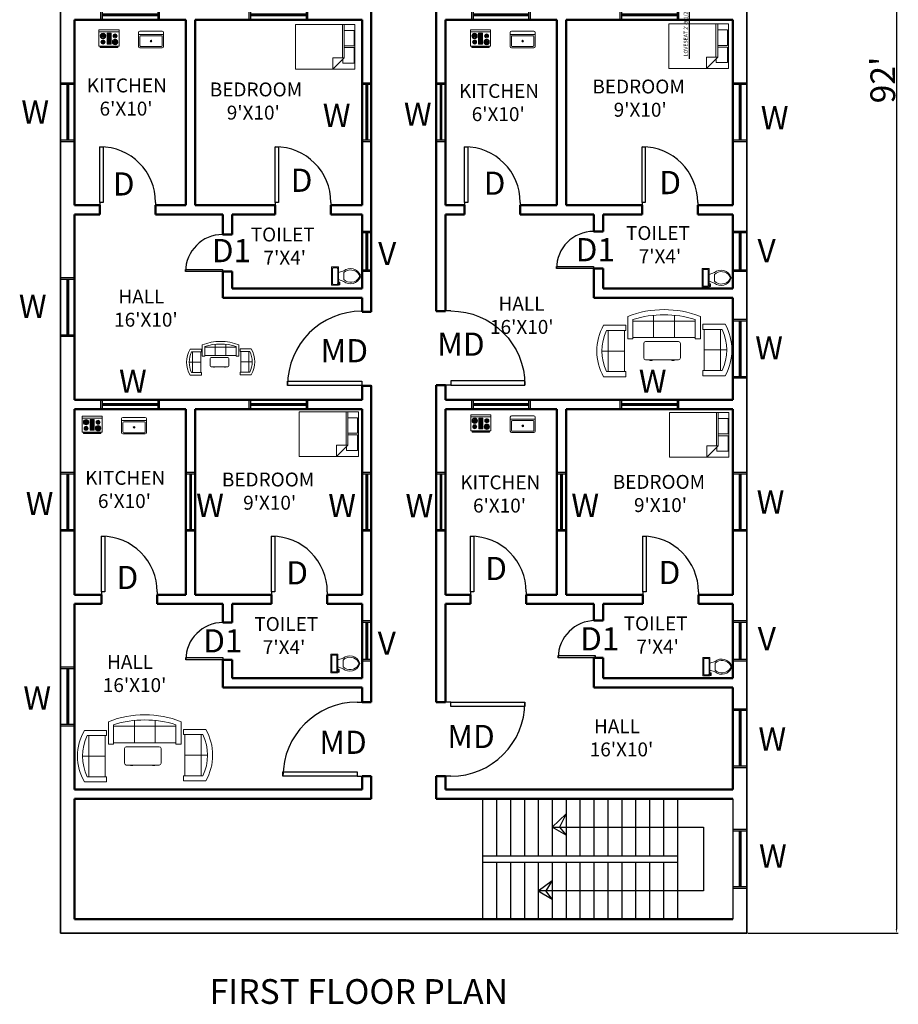
# Model space of a CAD drawing. Units: inches. Extents: x -25308 to -23933, y 10755 to 11996.
# Tile 1 of 6: x -25308 to -24739, y 10765 to 11402. Entities that reach past the tile are written whole.
import ezdxf

# ---------------------------------------------------------------- set-up
doc = ezdxf.new("R2010")
doc.units = ezdxf.units.IN
for name, color, linetype, lineweight in [('A-ANNO-DIMS', 2, 'Continuous', 18), ('A-ANNO-SYMB', 3, 'Continuous', 18), ('A-ANNO-TEXT', 7, 'Continuous', 25), ('A-AREA-IDEN', 7, 'Continuous', 18), ('A-DOOR', 3, 'Continuous', 25), ('A-FLOR-FIXT', 8, 'Continuous', 18), ('A-FLOR-STRS', 2, 'Continuous', 25), ('A-FURN', 8, 'Continuous', 18), ('A-GLAZ', 4, 'Continuous', 25), ('A-WALL', 7, 'Continuous', 50), ('C-PROP', 30, 'Continuous', 35)]:
    doc.layers.add(name, color=color, linetype=linetype, lineweight=lineweight)
doc.styles.get("Standard").update_dxf_attribs({"font": 'arial.ttf'})
doc.dimstyles.new('ISO-25', dxfattribs={"dimtxt": 2.5, "dimasz": 2.5, "dimexe": 1.25, "dimexo": 0.625, "dimtad": 1, "dimdec": 0, "dimlunit": 3, "dimtxsty": 'Standard', "dimcen": 2.5, "dimadec": 0, "dimazin": 0, "dimtfac": 1, "dimtdec": 0, "dimtmove": 0, "dimatfit": 3, "dimfxl": 1, "dimarcsym": 0})

# ---------------------------------------------------------------- blocks, each defined once
blk = doc.blocks.new('*U8')
for p, q in [((0, 0), (0, -100)), ((750, 0), (750, -100))]:
    blk.add_line(p, q)
blk.add_lwpolyline([(0, 0), (0, 750), (43.75, 750), (43.75, 0)], close=True)
blk.add_arc((0, 0), 750, 0, 90)
blk = doc.blocks.new('Desk - 30 x 60 in.')
for p, q in [((-26.999995, 0), (26.999995, 0)), ((-29.999995, -27), (-29.999995, -3)), ((29.999995, -3), (29.999995, -27)), ((26.999995, -30), (-26.999995, -30)), ((-20.000005, -30), (-20.000005, -31)), ((-20.000005, -31), (-16.000005, -31)), ((-16.000005, -31), (-16.000005, -30)), ((15.999995, -31), (15.999995, -30)), ((19.999995, -31), (15.999995, -31)), ((19.999995, -30), (19.999995, -31))]:
    blk.add_line(p, q)
for centre, start, end in [((-26.499995, -3.5), 98.1301, 171.8699), ((26.499995, -3.5), 8.130102, 81.8699), ((-26.499995, -26.5), 188.1301, 261.8699), ((26.499995, -26.5), 278.1301, 351.8699)]:
    blk.add_arc(centre, 3.535534, start, end)
blk = doc.blocks.new('Sofa - Roundback 7 ft.')
for p, q in [((-12.00002, -32.4421), (-12.00003, -6.5971)), ((11.99997, -32.4421), (11.99998, -6.5971)), ((-36.000027, -34), (-36.000027, -11.4696)), ((-35.999844, -13.3819), (35.9998, -13.3819)), ((35.99998, -34), (35.99998, -11.4696)), ((-36.000027, -32.4421), (35.99998, -32.4421))]:
    blk.add_line(p, q)
for points in [[(-36.000027, -34), (-42.000027, -34), (-42.000027, -8)], [(41.99998, -8), (41.99998, -34), (35.99998, -34)]]:
    blk.add_lwpolyline(points)
for centre, radius, start, end in [((0, -114.25), 114.25, 68.43141, 111.5686), ((-0.00001, -127.1968), 121.1968, 72.72033, 107.2797)]:
    blk.add_arc(centre, radius, start, end)
blk = doc.blocks.new('Sofa - Roundback Loveseat 5 ft.')
for p, q in [((-24, -33.99998), (-24, -11.46958)), ((0, -32.44198), (0, -5.99998)), ((24.00004, -33.99998), (24.00004, -11.46958)), ((-23.9998, -13.38178), (23.99986, -13.38178)), ((-24, -32.44198), (24.00004, -32.44198))]:
    blk.add_line(p, q)
for points in [[(-24, -33.99998), (-30, -33.99998), (-30, -7.99998)], [(30.00004, -7.99998), (30.00004, -33.99998), (24.00004, -33.99998)]]:
    blk.add_lwpolyline(points)
for centre, radius, start, end in [((0, -60.24998), 60.24998, 60.13715, 119.8628), ((0, -61.38438), 55.38444, 64.32083, 115.6792)]:
    blk.add_arc(centre, radius, start, end)
blk = doc.blocks.new('Bed - Queen')
for p, q in [((0, -80.00003), (0, 0)), ((0, 0), (59.99999, 0)), ((59.99999, 0), (59.99999, -80.00003)), ((7.99999, -1.2), (28.79998, -1.2)), ((7.99999, -14.4), (7.99999, -1.2)), ((28.79998, -1.2), (28.79998, -14.4)), ((31.19999, -1.2), (51.99999, -1.2)), ((31.19999, -14.4), (31.19999, -1.2)), ((51.99999, -1.2), (51.99999, -16.4)), ((0, -14.4), (44.8, -14.4)), ((44.8, -16.8), (0, -16.8)), ((59.99999, -29.6), (44.8, -14.4)), ((44.8, -14.4), (44.8, -29.6)), ((51.99999, -16.4), (46.79936, -16.4)), ((44.8, -29.6), (59.99999, -29.6)), ((59.99999, -80.00003), (0, -80.00003))]:
    blk.add_line(p, q)
blk = doc.blocks.new('Range-Oven - 30 in top')
for p, q in [((0, -3), (30, -3)), ((12, -6), (18, -6)), ((13, -20), (13, -6)), ((14, -6), (14, -20)), ((15, -20), (15, -6)), ((16, -6), (16, -20)), ((17, -20), (17, -6)), ((6, -24), (6, -25)), ((8, -25), (8, -24)), ((18, -20), (12, -20)), ((22, -25), (22, -24)), ((24, -24), (24, -25))]:
    blk.add_line(p, q)
for points in [[(0, -24), (0, 0), (30, 0), (30, -24)], [(12, -21), (12, -5), (18, -5), (18, -21)], [(2, -26), (2, -25), (28, -25), (28, -26)]]:
    blk.add_lwpolyline(points, close=True)
for centre, radius in [((6, -9), 4), ((6, -9), 3), ((6, -9), 2), ((6, -9), 1), ((24, -18), 4), ((24, -9), 3), ((24, -9), 2), ((24, -9), 1), ((6, -18), 3), ((6, -18), 2), ((6, -18), 1), ((24, -18), 3), ((24, -18), 2), ((24, -18), 1)]:
    blk.add_circle(centre, radius)
blk = doc.blocks.new('Sink-single - 30 in top')
blk.add_line((-15, -3.999996), (15, -3.999996))
for points in [[(-13.5, 0), (13.5, 0)], [(-15, -18.499996), (-15, -1.5)], [(-13.5, -17.499996), (-13.5, -6.499996)], [(-12.5, -5.499996), (12.5, -5.499996)], [(13.5, -6.499996), (13.5, -17.499996)], [(15, -1.5), (15, -18.499996)], [(13.5, -19.999996), (-13.5, -19.999996)], [(12.5, -18.499996), (-12.5, -18.499996)]]:
    blk.add_lwpolyline(points)
for radius in [1, 0.5]:
    blk.add_circle((0, -11.999996), radius)
for centre, radius, start, end in [((-13.5, -1.5), 1.5, 90, 180), ((-12.5, -6.499996), 1, 90, 180), ((12.5, -6.499996), 1, 0, 90), ((13.5, -1.5), 1.5, 0, 90), ((-13.5, -18.499996), 1.5, 180, 270), ((-12.5, -17.499996), 1, 180, 270), ((12.5, -17.499996), 1, 270, 0), ((13.5, -18.499996), 1.5, 270, 0)]:
    blk.add_arc(centre, radius, start, end)
blk = doc.blocks.new('Toilet - top')
for p, q in [((-10, -8.5), (-8, -8.5)), ((-10, -9.5), (-10, -8.5)), ((-7, -9.5), (-10, -9.5)), ((-8, -8.5), (-8, -8)), ((-7, -8), (-7, -9.5)), ((-4, -8), (-6, -14)), ((4, -8), (6, -14)), ((9.5, -6), (9.5, -2)), ((4, -14), (-4, -14))]:
    blk.add_line(p, q)
blk.add_lwpolyline([(10.5, -8), (10.5, 0), (-10.5, 0), (-10.5, -8)], close=True)
for points in [[(-9.5, -2), (-9.5, -6)], [(8.5, -1), (-8.5, -1)], [(-8.5, -7), (8.5, -7)]]:
    blk.add_lwpolyline(points)
for centre, radius, start, end in [((-8.6, -1.9), 0.884, 81.8699, 188.1301), ((-8.6, -6.1), 0.884, 171.8699, 278.1301), ((8.6, -1.9), 0.884, 351.8699, 98.1301), ((8.6, -6.1), 0.884, 261.8699, 8.1301), ((3.5, -21.6), 12.2, 141.4691, 247.9714), ((4.2, -21.8), 11.3, 136.3677, 238.9468), ((-3.5, -21.6), 12.2, 292.0284, 38.5307), ((-4.2, -21.8), 11.3, 301.053, 43.6321), ((0, -27.9), 4, 245.7318, 294.2682), ((0, -29), 4, 254.8605, 285.1395)]:
    blk.add_arc(centre, radius, start, end)
blk = doc.blocks.new('*D161')
at = {"layer": 'A-ANNO-DIMS', "color": 0, "lineweight": -2, "transparency": 16777216}
for p, q in [((-24836.82, 11915.12), (-24739.49, 11915.12)), ((-24740.74, 11912.62), (-24740.74, 10813.62)), ((-24836.82, 10811.12), (-24739.49, 10811.12))]:
    blk.add_line(p, q, dxfattribs=at)
at = {"layer": 'A-ANNO-DIMS', "color": 0, "transparency": 16777216}
for points in [[(-24741.15, 11912.62), (-24740.32, 11912.62), (-24740.74, 11915.12)], [(-24741.15, 10813.62), (-24740.32, 10813.62), (-24740.74, 10811.12)]]:
    blk.add_solid(points, dxfattribs=at)
at = {"layer": 'Defpoints', "color": 0, "transparency": 16777216}
for p in [(-24837.44, 11915.12), (-24837.44, 10811.12), (-24740.74, 10811.12)]:
    blk.add_point(p, dxfattribs=at)
at = {"layer": 'A-ANNO-DIMS', "color": 0, "transparency": 16777216, "insert": (-24749.53, 11363.12), "char_height": 2.5, "attachment_point": 5, "rotation": 90}
blk.add_mtext("{\\H6.4x;92'}", dxfattribs=at)
blk = doc.blocks.new('WIN-36-9IN')
for p, q in [((0, 9), (0, 0)), ((1, 9), (1, 0)), ((37, 9), (37, 0)), ((38, 9), (38, 0)), ((1, 5), (37, 5)), ((1, 4.5), (37, 4.5)), ((1, 4), (37, 4))]:
    blk.add_line(p, q)
blk = doc.blocks.new('VENT-24')
for p, q in [((0, 26), (9, 26)), ((0, 25), (9, 25)), ((4, 1), (4, 25)), ((4.5, 1), (4.5, 25)), ((5, 1), (5, 25)), ((0, 1), (9, 1)), ((0, 0), (9, 0))]:
    blk.add_line(p, q)
blk = doc.blocks.new('WIN-24-6IN')
for p, q in [((0, 26), (6, 26)), ((0, 25), (6, 25)), ((2.5, 1), (2.5, 25)), ((3, 1), (3, 25)), ((3.5, 1), (3.5, 25)), ((0, 1), (6, 1)), ((0, 0), (6, 0))]:
    blk.add_line(p, q)
blk = doc.blocks.new('WIN-36-6IN')
for p, q in [((0, 6), (0, 0)), ((1, 6), (1, 0)), ((1, 3.5), (37, 3.5)), ((1, 3), (37, 3)), ((1, 2.5), (37, 2.5)), ((37, 6), (37, 0)), ((38, 6), (38, 0))]:
    blk.add_line(p, q)
blk = doc.blocks.new('*D190')
at = {"layer": 'A-ANNO-DIMS', "color": 0, "lineweight": -2, "transparency": 16777216}
for p, q in [((-24870.41, 11454.17), (-24876.03, 11454.17)), ((-24874.78, 11451.67), (-24874.78, 11423.35)), ((-24870.41, 11420.85), (-24876.03, 11420.85)), ((-24874.78, 11420.85), (-24874.78, 11376.73))]:
    blk.add_line(p, q, dxfattribs=at)
at = {"layer": 'A-ANNO-DIMS', "color": 0, "transparency": 16777216}
for points in [[(-24875.2, 11451.67), (-24874.36, 11451.67), (-24874.78, 11454.17)], [(-24875.2, 11423.35), (-24874.36, 11423.35), (-24874.78, 11420.85)]]:
    blk.add_solid(points, dxfattribs=at)
at = {"layer": 'Defpoints', "color": 0, "transparency": 16777216}
for p in [(-24869.78, 11454.17), (-24874.78, 11420.85), (-24869.78, 11420.85)]:
    blk.add_point(p, dxfattribs=at)
at = {"layer": 'A-ANNO-DIMS', "color": 0, "transparency": 16777216, "insert": (-24876.7, 11397.54), "char_height": 2.5, "attachment_point": 5, "rotation": 90}
blk.add_mtext('LOVESEAT 2\'-9 1/2" TYP.', dxfattribs=at)

msp = doc.modelspace()

# ---------------------------------------------------------------- linework, layer by layer
at = {"layer": 'A-FLOR-STRS'}
for p, q in [((-25008.44, 10898.12), (-25008.44, 10820.12)), ((-24999.44, 10898.12), (-24999.44, 10861.12)), ((-24990.44, 10898.12), (-24990.44, 10861.12)), ((-24981.44, 10898.12), (-24981.44, 10861.12)), ((-24972.44, 10898.12), (-24972.44, 10861.12)), ((-24963.44, 10898.12), (-24963.44, 10861.12)), ((-24954.44, 10898.12), (-24954.44, 10861.12)), ((-24945.44, 10898.12), (-24945.44, 10861.12)), ((-24936.44, 10898.12), (-24936.44, 10861.12)), ((-24927.44, 10898.12), (-24927.44, 10861.12)), ((-24918.44, 10898.12), (-24918.44, 10861.12)), ((-24909.44, 10898.12), (-24909.44, 10861.12)), ((-24900.44, 10898.12), (-24900.44, 10861.12)), ((-24891.44, 10898.12), (-24891.44, 10861.12)), ((-24882.44, 10898.12), (-24882.44, 10820.12)), ((-24846.44, 10898.12), (-24846.44, 10820.12)), ((-24963.44, 10879.62), (-24954.44, 10888.37)), ((-24954.44, 10888.37), (-24958.64, 10879.62)), ((-24963.44, 10879.62), (-24865.43, 10879.62)), ((-24954.44, 10874.42), (-24963.44, 10879.62)), ((-24958.64, 10879.62), (-24954.44, 10874.42)), ((-24865.43, 10879.62), (-24865.43, 10838.62)), ((-25008.44, 10861.12), (-24882.44, 10861.12)), ((-25008.44, 10857.12), (-24882.44, 10857.12)), ((-24999.44, 10857.12), (-24999.44, 10820.12)), ((-24990.44, 10857.12), (-24990.44, 10820.12)), ((-24981.44, 10857.12), (-24981.44, 10820.12)), ((-24972.44, 10857.12), (-24972.44, 10820.12)), ((-24963.44, 10857.12), (-24963.44, 10820.12)), ((-24954.44, 10857.12), (-24954.44, 10820.12)), ((-24945.44, 10857.12), (-24945.44, 10820.12)), ((-24936.44, 10857.12), (-24936.44, 10820.12)), ((-24927.44, 10857.12), (-24927.44, 10820.12)), ((-24918.44, 10857.12), (-24918.44, 10820.12)), ((-24909.44, 10857.12), (-24909.44, 10820.12)), ((-24900.44, 10857.12), (-24900.44, 10820.12)), ((-24891.44, 10857.12), (-24891.44, 10820.12)), ((-24972.44, 10838.62), (-24963.44, 10845.13)), ((-24963.44, 10845.13), (-24967.58, 10838.62)), ((-24865.43, 10838.62), (-24972.44, 10838.62)), ((-24972.44, 10838.62), (-24963.44, 10833.02)), ((-24963.44, 10833.02), (-24967.58, 10838.62))]:
    msp.add_line(p, q, dxfattribs=at)
at = {"layer": 'A-WALL'}
for p, q in [((-25080.44, 11213.16), (-25080.44, 11416.06)), ((-25038.44, 11416.36), (-25038.44, 11213.64)), ((-25272.44, 11402.12), (-25200.44, 11402.12)), ((-25272.44, 11282.12), (-25272.44, 11402.12)), ((-25200.44, 11282.12), (-25200.44, 11402.12)), ((-25194.44, 11282.12), (-25194.44, 11402.12)), ((-25194.44, 11402.12), (-25086.44, 11402.12)), ((-25086.44, 11282.12), (-25086.44, 11402.12)), ((-25032.44, 11402.12), (-24960.44, 11402.12)), ((-25032.44, 11402.12), (-25032.44, 11282.12)), ((-24960.44, 11402.12), (-24960.44, 11282.12)), ((-24954.44, 11402.12), (-24954.44, 11282.12)), ((-24954.44, 11402.12), (-24846.44, 11402.12)), ((-24846.44, 11402.12), (-24846.44, 11282.12)), ((-25272.44, 11282.12), (-25256.02, 11282.12)), ((-25256.02, 11282.12), (-25256.02, 11276.12)), ((-25220.02, 11282.12), (-25220.02, 11276.12)), ((-25220.02, 11282.12), (-25200.44, 11282.12)), ((-25194.44, 11282.12), (-25142.59, 11282.12)), ((-25142.59, 11282.12), (-25142.59, 11276.12)), ((-25106.59, 11282.12), (-25106.59, 11276.12)), ((-25106.59, 11282.12), (-25086.44, 11282.12)), ((-25032.44, 11282.12), (-25020.09, 11282.12)), ((-25020.09, 11282.12), (-25020.09, 11276.12)), ((-24984.09, 11282.12), (-24984.09, 11276.12)), ((-24984.09, 11282.12), (-24960.44, 11282.12)), ((-24954.44, 11282.12), (-24905.28, 11282.12)), ((-24905.28, 11282.12), (-24905.28, 11276.12)), ((-24869.28, 11282.12), (-24869.28, 11276.12)), ((-24869.28, 11282.12), (-24846.44, 11282.12)), ((-25272.44, 11276.12), (-25256.02, 11276.12)), ((-25272.44, 11156.12), (-25272.44, 11276.12)), ((-25220.02, 11276.12), (-25176.44, 11276.12)), ((-25176.44, 11263.13), (-25176.44, 11276.12)), ((-25176.44, 11263.13), (-25176.44, 11276.12)), ((-25170.44, 11276.12), (-25142.59, 11276.12)), ((-25170.44, 11263.13), (-25170.44, 11276.12)), ((-25170.44, 11263.13), (-25170.44, 11276.12)), ((-25106.59, 11276.12), (-25086.44, 11276.12)), ((-25086.44, 11228.12), (-25086.44, 11276.12)), ((-25032.44, 11276.12), (-25020.09, 11276.12)), ((-25032.44, 11276.12), (-25032.44, 11213.64)), ((-24984.09, 11276.12), (-24936.44, 11276.12)), ((-24936.44, 11276.12), (-24936.44, 11265.12)), ((-24936.44, 11276.12), (-24936.44, 11265.12)), ((-24930.44, 11276.12), (-24930.44, 11265.12)), ((-24930.44, 11276.12), (-24930.44, 11265.12)), ((-24930.44, 11276.12), (-24905.28, 11276.12)), ((-24869.28, 11276.12), (-24846.44, 11276.12)), ((-24846.44, 11276.12), (-24846.44, 11228.12)), ((-25176.44, 11263.13), (-25170.44, 11263.13)), ((-24936.44, 11265.12), (-24930.44, 11265.12)), ((-25176.44, 11222.12), (-25176.44, 11239.13)), ((-25176.44, 11222.12), (-25176.44, 11239.13)), ((-25176.44, 11239.13), (-25170.44, 11239.13)), ((-25170.44, 11228.12), (-25170.44, 11239.13)), ((-25170.44, 11228.12), (-25170.44, 11239.13)), ((-24936.44, 11241.12), (-24930.44, 11241.12)), ((-24936.44, 11241.12), (-24936.44, 11222.12)), ((-24936.44, 11241.12), (-24936.44, 11222.12)), ((-24930.44, 11241.12), (-24930.44, 11228.12)), ((-24930.44, 11241.12), (-24930.44, 11228.12)), ((-25170.44, 11228.12), (-25086.44, 11228.12)), ((-24930.44, 11228.12), (-24846.44, 11228.12)), ((-25176.44, 11222.12), (-25086.44, 11222.12)), ((-25086.44, 11213.16), (-25086.44, 11222.12)), ((-24936.44, 11222.12), (-24846.44, 11222.12)), ((-24846.44, 11222.12), (-24846.44, 11156.12)), ((-25086.44, 11213.16), (-25080.44, 11213.16)), ((-25038.44, 11213.64), (-25032.44, 11213.64)), ((-25086.44, 11156.12), (-25086.44, 11165.16)), ((-25086.44, 11165.16), (-25080.44, 11165.16)), ((-25080.44, 10960.62), (-25080.44, 11165.16)), ((-25038.44, 11165.64), (-25032.44, 11165.64)), ((-25038.44, 11165.64), (-25038.44, 10960.62)), ((-25032.44, 11165.64), (-25032.44, 11156.12)), ((-25272.44, 11156.12), (-25176.44, 11156.12)), ((-25176.44, 11156.12), (-25086.44, 11156.12)), ((-25032.44, 11156.12), (-24846.44, 11156.12)), ((-25272.44, 11150.12), (-25200.44, 11150.12)), ((-25272.44, 11030.12), (-25272.44, 11150.12)), ((-25200.44, 11030.12), (-25200.44, 11150.12)), ((-25194.44, 11030.12), (-25194.44, 11150.12)), ((-25194.44, 11150.12), (-25086.44, 11150.12)), ((-25086.44, 11030.12), (-25086.44, 11150.12)), ((-25032.44, 11150.12), (-24960.44, 11150.12)), ((-25032.44, 11150.12), (-25032.44, 11030.12)), ((-24960.44, 11150.12), (-24960.44, 11030.12)), ((-24954.44, 11150.12), (-24954.44, 11030.12)), ((-24954.44, 11150.12), (-24846.44, 11150.12)), ((-24846.44, 11150.12), (-24846.44, 11030.12)), ((-25272.44, 11030.12), (-25254.98, 11030.12)), ((-25254.98, 11030.12), (-25254.98, 11024.12)), ((-25218.98, 11030.12), (-25218.98, 11024.12)), ((-25218.98, 11030.12), (-25200.44, 11030.12)), ((-25194.44, 11030.12), (-25144.93, 11030.12)), ((-25144.93, 11030.12), (-25144.93, 11024.12)), ((-25108.93, 11030.12), (-25108.93, 11024.12)), ((-25108.93, 11030.12), (-25086.44, 11030.12)), ((-25032.44, 11030.12), (-25016.19, 11030.12)), ((-25016.19, 11030.12), (-25016.19, 11024.12)), ((-24980.19, 11030.12), (-24980.19, 11024.12)), ((-24980.19, 11030.12), (-24960.44, 11030.12)), ((-24954.44, 11030.12), (-24904.78, 11030.12)), ((-24904.78, 11030.12), (-24904.78, 11024.12)), ((-24868.78, 11030.12), (-24868.78, 11024.12)), ((-24868.78, 11030.12), (-24846.44, 11030.12)), ((-25272.44, 11024.12), (-25254.98, 11024.12)), ((-25272.44, 10904.12), (-25272.44, 11024.12)), ((-25218.98, 11024.12), (-25176.44, 11024.12)), ((-25176.44, 11012.07), (-25176.44, 11024.12)), ((-25170.44, 11024.12), (-25144.93, 11024.12)), ((-25170.44, 11012.07), (-25170.44, 11024.12)), ((-25108.93, 11024.12), (-25086.44, 11024.12)), ((-25086.44, 10976.12), (-25086.44, 11024.12)), ((-25032.44, 11024.12), (-25016.19, 11024.12)), ((-25032.44, 11024.12), (-25032.44, 10960.62)), ((-24980.19, 11024.12), (-24936.44, 11024.12)), ((-24936.44, 11024.12), (-24936.44, 11013.36)), ((-24930.44, 11024.12), (-24930.44, 11013.36)), ((-24930.44, 11024.12), (-24904.78, 11024.12)), ((-24868.78, 11024.12), (-24846.44, 11024.12)), ((-24846.44, 11024.12), (-24846.44, 10976.12)), ((-25176.44, 11012.07), (-25170.44, 11012.07)), ((-24936.44, 11013.36), (-24930.44, 11013.36)), ((-24936.44, 10989.36), (-24930.44, 10989.36)), ((-24936.44, 10989.36), (-24936.44, 10970.12)), ((-24930.44, 10989.36), (-24930.44, 10976.12)), ((-25176.44, 10970.12), (-25176.44, 10988.07)), ((-25176.44, 10988.07), (-25170.44, 10988.07)), ((-25170.44, 10976.12), (-25170.44, 10988.07)), ((-25170.44, 10976.12), (-25086.44, 10976.12)), ((-24930.44, 10976.12), (-24846.44, 10976.12)), ((-25176.44, 10970.12), (-25086.44, 10970.12)), ((-25086.44, 10960.62), (-25086.44, 10970.12)), ((-24936.44, 10970.12), (-24846.44, 10970.12)), ((-24846.44, 10970.12), (-24846.44, 10904.12)), ((-25086.44, 10960.62), (-25080.44, 10960.62)), ((-25038.44, 10960.62), (-25032.44, 10960.62)), ((-25086.44, 10904.12), (-25086.44, 10912.62)), ((-25086.44, 10912.62), (-25080.44, 10912.62)), ((-25080.44, 10898.12), (-25080.44, 10912.62)), ((-25038.44, 10912.62), (-25032.44, 10912.62)), ((-25038.44, 10912.62), (-25038.44, 10898.12)), ((-25032.44, 10912.62), (-25032.44, 10904.12)), ((-25272.44, 10904.12), (-25086.44, 10904.12)), ((-25032.44, 10904.12), (-24846.44, 10904.12)), ((-25272.44, 10820.12), (-25272.44, 10898.12)), ((-25272.44, 10898.12), (-25080.44, 10898.12)), ((-25038.44, 10898.12), (-24846.44, 10898.12)), ((-24846.44, 10820.12), (-25272.44, 10820.12))]:
    msp.add_line(p, q, dxfattribs=at)
at = {"layer": 'C-PROP'}
for p, q in [((-25281.44, 10811.12), (-25281.44, 11915.12)), ((-24837.44, 11915.12), (-24837.44, 10811.12)), ((-24837.44, 10811.12), (-25281.44, 10811.12))]:
    msp.add_line(p, q, dxfattribs=at)

# ---------------------------------------------------------------- block references
at = {"layer": 'A-DOOR', "xscale": 0.0480000000000013, "yscale": 0.0480000000000013, "zscale": 0.0480000000000013}
for p in [(-25256.02, 11283.92), (-25142.59, 11283.92), (-25020.09, 11283.92), (-24905.28, 11283.92), (-25254.98, 11031.92), (-25144.93, 11031.92), (-25016.19, 11031.92), (-24904.78, 11031.92)]:
    msp.add_blockref('*U8', p, dxfattribs=at)
at = {"layer": 'A-DOOR'}
for p, xscale, yscale, zscale, rotation in [((-25176.62, 11239.14), 0.0320000000000009, 0.0320000000000009, 0.0320000000000009, 90), ((-24936.64, 11241.11), 0.0320000000000009, 0.0320000000000009, 0.0320000000000009, 90), ((-25086.6, 11165.52), 0.0640305237838995, 0.0640305237838995, 0.0640305237838995, 90), ((-25029.04, 11165.64), -0.0640305237838995, 0.0640305237838995, 0.0640305237838995, 270), ((-25176.44, 10988.07), 0.0320000000000009, 0.0320000000000009, 0.0320000000000009, 90), ((-24935.52, 10989.36), 0.0320000000000009, 0.0320000000000009, 0.0320000000000009, 90), ((-25089.54, 10912.6), 0.0640725944084254, 0.0640725944084254, 0.0640725944084254, 90), ((-25029.04, 10960.62), 0.0639999974380737, 0.0639999974380737, 0.0639999974380737, 270)]:
    msp.add_blockref('*U8', p, dxfattribs=dict(at, xscale=xscale, yscale=yscale, zscale=zscale, rotation=rotation))
at = {"layer": 'A-FLOR-FIXT'}
for name, p, xscale, yscale, zscale in [('Range-Oven - 30 in top', (-25256.64, 11395.48), 0.4338097128947254, 0.4338097128947254, 0.4338097128947254), ('Sink-single - 30 in top', (-25222.96, 11394.71), 0.5374838416175965, 0.5374838416175965, 0.5374838416175965), ('Range-Oven - 30 in top', (-25016.25, 11395.48), 0.4338097128947254, 0.4338097128947254, 0.4338097128947254), ('Sink-single - 30 in top', (-24982.57, 11394.71), 0.5374838416175965, 0.5374838416175965, 0.5374838416175965), ('Range-Oven - 30 in top', (-25267.61, 11145.62), 0.4338097128947254, 0.4338097128947254, 0.4338097128947254), ('Sink-single - 30 in top', (-25233.93, 11144.85), 0.5374838416175965, 0.5374838416175965, 0.5374838416175965), ('Range-Oven - 30 in top', (-25016.13, 11146.55), 0.4338097128947254, 0.4338097128947254, 0.4338097128947254), ('Sink-single - 30 in top', (-24982.45, 11145.78), 0.5374838416175965, 0.5374838416175965, 0.5374838416175965)]:
    msp.add_blockref(name, p, dxfattribs=dict(at, xscale=xscale, yscale=yscale, zscale=zscale))
at = {"layer": 'A-FLOR-FIXT', "xscale": 0.5659332238665749, "yscale": 0.5659332238665749, "zscale": 0.5659332238665749, "rotation": 90}
for p in [(-25106.15, 11236.21), (-24866.36, 11235.11), (-25106.64, 10985.6), (-24865.9, 10983.53)]:
    msp.add_blockref('Toilet - top', p, dxfattribs=at)
at = {"layer": 'A-FURN'}
for name, p, xscale, yscale, zscale, rotation in [('Bed - Queen', (-25091.03, 11399.04), 0.4812808282186369, 0.4812808282186369, 0.4812808282186369, 270), ('Bed - Queen', (-24849.37, 11399.35), 0.4812808282186369, 0.4812808282186369, 0.4812808282186369, 270), ('Sofa - Roundback Loveseat 5 ft.', (-24934.58, 11187.77), 0.5553292889469988, 0.5553292889469988, 0.5553292889469988, 89.99999999999999), ('Sofa - Roundback Loveseat 5 ft.', (-24847.12, 11188.42), 0.5553292889469988, 0.5553292889469988, 0.5553292889469988, 270), ('Sofa - Roundback Loveseat 5 ft.', (-25199.93, 11180.48), 0.2798473955820579, 0.2798473955820579, 0.2798473955820579, 89.99999999999999), ('Sofa - Roundback Loveseat 5 ft.', (-25155.86, 11180.81), 0.2798473955820579, 0.2798473955820579, 0.2798473955820579, 270), ('Bed - Queen', (-25088.71, 11148.46), 0.4812808282186369, 0.4812808282186369, 0.4812808282186369, 270), ('Bed - Queen', (-24849.08, 11147.95), 0.4812808282186369, 0.4812808282186369, 0.4812808282186369, 270), ('Sofa - Roundback Loveseat 5 ft.', (-25270.55, 10925.64), 0.5553292889469988, 0.5553292889469988, 0.5553292889469988, 89.99999999999999), ('Sofa - Roundback Loveseat 5 ft.', (-25183.09, 10926.28), 0.5553292889469988, 0.5553292889469988, 0.5553292889469988, 270)]:
    msp.add_blockref(name, p, dxfattribs=dict(at, xscale=xscale, yscale=yscale, zscale=zscale, rotation=rotation))
for name, p, xscale, yscale, zscale in [('Sofa - Roundback 7 ft.', (-24891.06, 11214.57), 0.559663641165008, 0.559663641165008, 0.559663641165008), ('Sofa - Roundback 7 ft.', (-25178, 11193.99), 0.2820316080914415, 0.2820316080914415, 0.2820316080914415), ('Desk - 30 x 60 in.', (-24892.36, 11193.91), 0.3949565101416468, 0.3949565101416468, 0.3949565101416468), ('Desk - 30 x 60 in.', (-25178.66, 11183.58), 0.1990306524997052, 0.1990306524997052, 0.1990306524997052), ('Sofa - Roundback 7 ft.', (-25227.03, 10952.43), 0.559663641165008, 0.559663641165008, 0.559663641165008), ('Desk - 30 x 60 in.', (-25228.33, 10931.77), 0.3949565101416468, 0.3949565101416468, 0.3949565101416468)]:
    msp.add_blockref(name, p, dxfattribs=dict(at, xscale=xscale, yscale=yscale, zscale=zscale))
at = {"layer": 'A-GLAZ'}
for name, p, rotation in [('WIN-36-6IN', (-25217.44, 11408.12), 180), ('WIN-36-6IN', (-25121.44, 11408.12), 180), ('WIN-36-6IN', (-24977.44, 11408.12), 180), ('WIN-36-6IN', (-24881.44, 11408.12), 180), ('WIN-36-9IN', (-25281.44, 11361.12), 270.0000000000339), ('WIN-36-6IN', (-25086.44, 11361.12), 270.0000000000161), ('WIN-36-6IN', (-25038.44, 11361.12), 270.0000000000268), ('WIN-36-9IN', (-24846.44, 11361.12), 270.0000000000198), ('WIN-24-6IN', (-25080.44, 11265.12), 180), ('VENT-24', (-24837.44, 11265.12), 180), ('VENT-24', (-24837.44, 11265.12), 180), ('WIN-36-9IN', (-25281.44, 11235.12), 270.0000000000315), ('WIN-36-9IN', (-24846.44, 11208.12), 270.0000000000173), ('WIN-36-6IN', (-25217.44, 11156.12), 180), ('WIN-36-6IN', (-25121.44, 11156.12), 180), ('WIN-36-6IN', (-24977.44, 11156.12), 180), ('WIN-36-6IN', (-24881.44, 11156.12), 180), ('WIN-36-9IN', (-25281.44, 11109.12), 270.0000000000339), ('WIN-36-6IN', (-25200.44, 11109.12), 270.0000000000268), ('WIN-36-6IN', (-25086.44, 11109.12), 270.0000000000143), ('WIN-36-6IN', (-25038.44, 11109.12), 270.0000000000161), ('WIN-36-6IN', (-24960.44, 11109.12), 270.0000000000161), ('WIN-36-9IN', (-24846.44, 11109.12), 270.0000000000211), ('WIN-24-6IN', (-25080.44, 11013.12), 180), ('VENT-24', (-24837.44, 11013.12), 180), ('VENT-24', (-24837.44, 11013.12), 180), ('WIN-36-9IN', (-25281.44, 10983.12), 270.0000000000277), ('WIN-36-9IN', (-24846.44, 10956.12), 270.0000000000211), ('WIN-36-9IN', (-24846.44, 10878.12), 270.0000000000094)]:
    msp.add_blockref(name, p, dxfattribs=dict(at, rotation=rotation))

# ---------------------------------------------------------------- texts
at = {"layer": 'A-ANNO-SYMB', "char_height": 15, "attachment_point": 1}
for s, insert in [('{W}', (-25306.89, 11349.92)), ('{W}', (-25111.84, 11347.71)), ('{W}', (-25059.37, 11348.51)), ('{W}', (-24828.46, 11346.19)), ('{D}', (-25247.71, 11303.35)), ('{D}', (-25132.61, 11305.73)), ('{D}', (-25007.75, 11303.81)), ('{D}', (-24894.13, 11304.24)), ('{D1}', (-25183.67, 11260.23)), ('{V}', (-25076.06, 11258.33)), ('{D1}', (-24948.23, 11260.81)), ('{V}', (-24830.59, 11260.14)), ('{W}', (-25308.47, 11224.22)), ('{MD}', (-25037.79, 11199.68)), ('{MD}', (-25113.25, 11195.47)), ('{W}', (-24832.1, 11197.34)), ('{W}', (-25243.69, 11175.71)), ('{W}', (-24907.39, 11175.71)), ('{W}', (-24831.15, 11097.62)), ('{W}', (-25304.07, 11096.65)), ('{W}', (-25193.79, 11095.46)), ('{W}', (-25108.33, 11095.34)), ('{W}', (-25058.33, 11095.19)), ('{W}', (-24951.06, 11095.44)), ('{D}', (-25006.79, 11054.56)), ('{D}', (-25245.3, 11048.73)), ('{D}', (-25135.49, 11051.78)), ('{D}', (-24894.56, 11051.92)), ('{D1}', (-25189.21, 11007.77)), ('{D1}', (-24945.37, 11009.06)), ('{V}', (-24830.43, 11009.14)), ('{V}', (-25076.32, 11006.23)), ('{W}', (-25305.61, 10970.83)), ('{MD}', (-25031.27, 10945.87)), ('{W}', (-24830.01, 10944.26)), ('{MD}', (-25114.09, 10942.11)), ('{W}', (-24829.63, 10868.49))]:
    msp.add_mtext_dynamic_manual_height_columns(s, width=1123.2502, gutter_width=12.5, heights=[0], dxfattribs=dict(at, insert=insert))
at = {"layer": 'A-ANNO-TEXT', "insert": (-25185.06, 10781.38), "char_height": 16, "attachment_point": 1}
msp.add_mtext_dynamic_manual_height_columns('{FIRST FLOOR PLAN}', width=693.9138, gutter_width=12.5, heights=[0], dxfattribs=at)
at = {"layer": 'A-AREA-IDEN', "char_height": 9, "attachment_point": 1}
for s, heights, insert in [("{KITCHEN\\P   6'X10'}", [0], (-25264.52, 11364.08)), ("{BEDROOM\\P    9'X10'}", [0], (-25184.95, 11361.49)), ("{KITCHEN\\P   6'X10'}", [0], (-25023.73, 11360.53)), ("{BEDROOM\\P     9'X10'}", [0], (-24937.38, 11363.37)), ("{TOILET\\P   7'X4'}", [24.16], (-25158.44, 11267.64)), ("{TOILET\\P   7'X4'}", [0], (-24915.69, 11268.6)), ("{     HALL\\P    16'X10'}", [0], (-25257.83, 11227.52)), ("{        HALL\\P      16'X10' }", [0], (-25020.14, 11222.86)), ("{KITCHEN\\P   6'X10'}", [0], (-25265.57, 11110.2)), ("{BEDROOM\\P     9'X10'}", [0], (-25177.11, 11109.11)), ("{KITCHEN\\P   6'X10'}", [0], (-25022.89, 11107.27)), ("{BEDROOM\\P     9'X10'}", [0], (-24924.24, 11107.59)), ("{TOILET\\P  7'X4'}", [0], (-25156.13, 11015.65)), ("{TOILET\\P   7'X4'}", [0], (-24917.19, 11016.02)), ("{     HALL\\P    16'X10'}", [0], (-25265.16, 10991.14)), ("{  HALL\\P 16'X10'}", [0], (-24941.89, 10949.5))]:
    msp.add_mtext_dynamic_manual_height_columns(s, width=1489.8169, gutter_width=12.5, heights=heights, dxfattribs=dict(at, insert=insert))

# ---------------------------------------------------------------- dimensions: what is measured, and where the dimension line sits
at = {"layer": 'A-ANNO-DIMS'}
for base, p1, p2, angle, text, override, picture, middle in [((-24740.74, 10811.12), (-24837.44, 11915.12), (-24837.44, 10811.12), 90, '{\\H6.4x;<>}', {"dimclrd": 0, "dimclre": 0, "dimclrt": 0}, '*D161', (-24749.53, 11363.12)), ((-24874.78, 11420.85), (-24869.78, 11454.17), (-24869.78, 11420.85), 270, 'LOVESEAT <> TYP.', {"dimdec": 1, "dimlfac": 1, "dimrnd": 0, "dimzin": 1, "dimdsep": 46, "dimlunit": 4, "dimfrac": 2}, '*D190', (-24876.7, 11397.54))]:
    dim = msp.add_linear_dim(base=base, p1=p1, p2=p2, angle=angle, text=text, dimstyle='ISO-25', override=override, dxfattribs=at)
    dim.commit()
    dim.dimension.update_dxf_attribs({"geometry": picture, "text_midpoint": middle})

doc.saveas('drawing.dxf')
